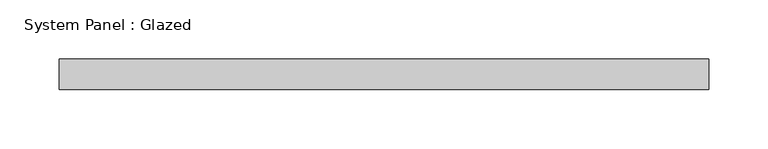
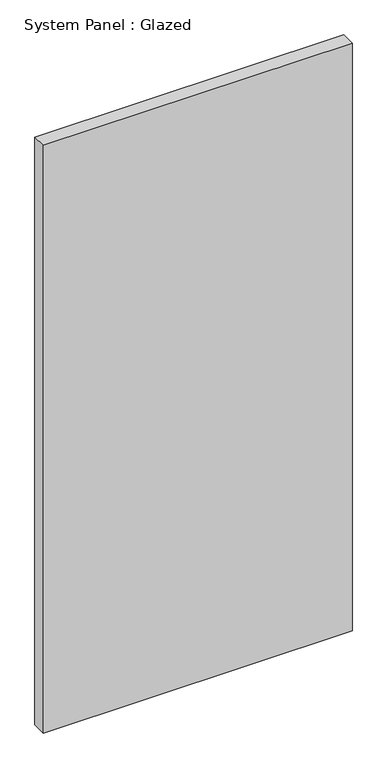
"""IFC4 building model written with IfcOpenShell, lengths in millimetres: plate geometry, System Panel : Glazed."""

from ifc_helpers import new_model, si_unit, origin, origin_with_axes, place, context, project, spatial, polyline, outline, extrude, source, transform, mapped, element, save


def system_panel_glazed_5eb04348(model_context):
    return source(origin(), model_context, "Body", "SweptSolid", [
        extrude(outline(polyline([(273.05, 19.05), (-273.05, 19.05), (-273.05, 44.45), (273.05, 44.45), (273.05, 19.05)])), origin_with_axes(), (0.0, 0.0, 1.0), 1098.55),
    ])


if __name__ == "__main__":
    model = new_model("IFC4")
    model_context = context("Model", 3, world=origin())
    ifc_project = project(units=[si_unit("LENGTHUNIT", "METRE", prefix="MILLI")], contexts=[model_context])
    site = spatial("IfcSite", under=ifc_project)
    building = spatial("IfcBuilding", under=site)
    placement = place(None, origin())
    system_panel_glazed_shape = system_panel_glazed_5eb04348(model_context)
    element("IfcPlate", 1, ObjectType="System Panel : Glazed", at=placement, inside=building, context=model_context, shape_type="MappedRepresentation", body=[
        mapped(system_panel_glazed_shape, transform((0.0, 0.0, 0.0), x_axis=(1.0, 0.0, 0.0), y_axis=(0.0, 1.0, 0.0), z_axis=(0.0, 0.0, 1.0))),
    ])
    save(model, "model.ifc")

# Revit data of these elements
# Type "System Panel : Glazed"
#   Construction Type Id = "GSP4R"
#   Analytic Construction = "1/8 in Pilkington single glazing"
#   Visual Light Transmittance = 0.9
#   Solar Heat Gain Coefficient = 0.86
#   Heat Transfer Coefficient (U) = 1.18115 BTU/(h·ft²·°F)
#   Define Thermal Properties by = 1
# Element 1 (IfcPlate, "System Panel : Glazed")
#   Materials on its faces: "Glass"
# Materials
#   "Glass": class "Glass", colour RGB 0 128 192, transparency 0.75, Description = "Soda Lime Glass", Cost = 0
